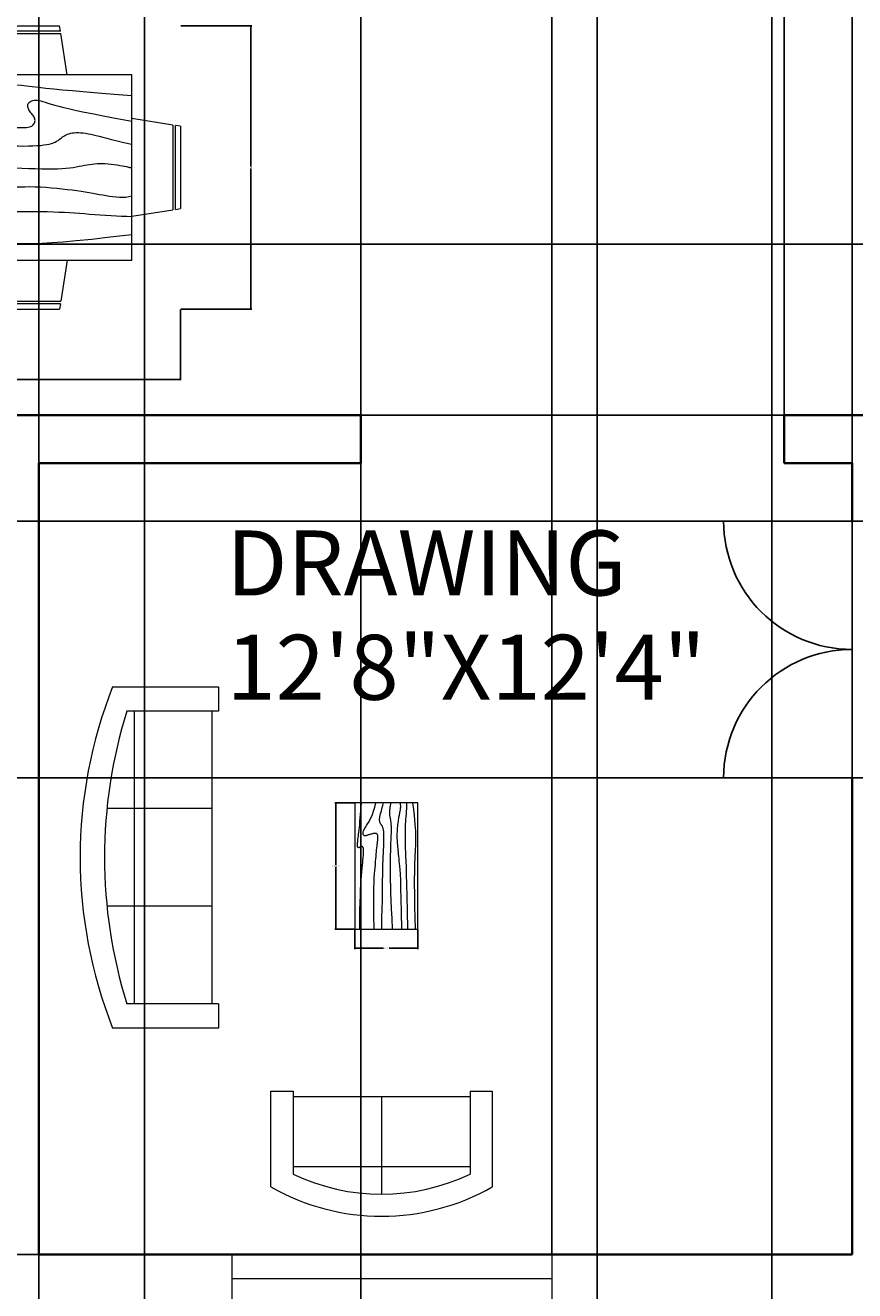
# Model space of a CAD drawing. Units: feet. Extents: x 2270 to 3094, y 1543 to 2352.
# Tile 4 of 6: x 2662 to 2817, y 1813 to 2050. Entities that reach past the tile are written whole.
import ezdxf

# ---------------------------------------------------------------- set-up
doc = ezdxf.new("R2010")
doc.units = ezdxf.units.FT
for name, color, linetype, lineweight in [('A-ANNO-DIMS', 2, 'Continuous', 18), ('A-AREA-IDEN', 7, 'Continuous', 18), ('A-DOOR', 3, 'Continuous', 25), ('A-FURN', 8, 'Continuous', 18), ('A-GLAZ', 4, 'Continuous', 18), ('A-WALL', 7, 'Continuous', 35)]:
    doc.layers.add(name, color=color, linetype=linetype, lineweight=lineweight)
doc.styles.get("Standard").update_dxf_attribs({"font": 'arial.ttf'})
doc.dimstyles.get("Standard").update_dxf_attribs({"dimtxt": 0.18, "dimasz": 0.18, "dimexe": 0.18, "dimexo": 0.0625, "dimgap": 0.09, "dimtad": 0, "dimtih": 1, "dimtoh": 1, "dimdec": 4, "dimzin": 0, "dimdsep": 46, "dimtxsty": 'Standard', "dimcen": 0.09, "dimadec": 0, "dimazin": 0, "dimtfac": 1, "dimtdec": 4, "dimtofl": 0, "dimtmove": 0, "dimatfit": 3, "dimfxl": 1, "dimtolj": 1, "dimtzin": 0, "dimarcsym": 0})

# ---------------------------------------------------------------- blocks, each defined once
blk = doc.blocks.new('Dining Set - 36 x 72 in.')
for p, q in [((-22, 27.5), (-22.1562, 26.50042)), ((-22, 27.5), (-6, 27.5)), ((-5.8437, 26.49966), (-6, 27.5)), ((6, 27.5), (5.8438, 26.50042)), ((6, 27.5), (22, 27.5)), ((22.1563, 26.49966), (22, 27.5)), ((-22.2343, 26.00059), (-23.4847, 17.99762)), ((-22.2304, 26), (-5.7608, 26)), ((-5.8416, 26.5), (-22.1534, 26.5)), ((-4.5152, 17.99762), (-5.7655, 25.99926)), ((5.7657, 26.00059), (4.5153, 17.99762)), ((5.7696, 26), (22.2392, 26)), ((22.1584, 26.5), (5.8466, 26.5)), ((23.4848, 17.99762), (22.2345, 25.99926)), ((36, 18), (-36, 18)), ((-36, 18), (-36, -18)), ((36, -18), (36, 18)), ((-45.5, 8), (-44.5004, 8.15617)), ((-45.5, 8), (-45.5, -8)), ((-44.5, -8.15843), (-44.5, 8.15338)), ((-44.0006, 8.23428), (-35.9976, 9.48474)), ((-44, 8.23041), (-44, -8.23915)), ((44.0006, 8.23428), (35.9976, 9.48474)), ((44, 8.23041), (44, -8.23915)), ((44.5, -8.15843), (44.5, 8.15338)), ((45.5, 8), (44.5005, 8.15617)), ((45.5, 8), (45.5, -8)), ((-44.4997, -8.15631), (-45.5, -8)), ((-35.9976, -9.48476), (-43.9993, -8.2345)), ((35.9976, -9.48476), (43.9993, -8.2345)), ((44.4997, -8.15631), (45.5, -8)), ((-36, -18), (36, -18)), ((-22.2343, -26.0006), (-23.4847, -17.99762)), ((-4.5152, -17.99762), (-5.7655, -25.99928)), ((5.7657, -26.0006), (4.5153, -17.99762)), ((23.4848, -17.99762), (22.2345, -25.99928)), ((-22.2304, -26), (-5.7608, -26)), ((-22, -27.5), (-22.1562, -26.50044)), ((-5.8416, -26.5), (-22.1534, -26.5)), ((-5.8437, -26.49967), (-6, -27.5)), ((5.7696, -26), (22.2392, -26)), ((6, -27.5), (5.8438, -26.50044)), ((22.1584, -26.5), (5.8466, -26.5)), ((22.1563, -26.49967), (22, -27.5)), ((-22, -27.5), (-6, -27.5)), ((6, -27.5), (22, -27.5))]:
    blk.add_line(p, q)
for points in [[(-36, 15), (-31.1772, 14.97754), (-26.8079, 14.91406), (-22.8538, 14.81543), (-19.276, 14.6875), (-16.0362, 14.53613), (-13.0957, 14.36718), (-10.4159, 14.18652), (-7.9583, 14), (-5.6904, 13.81315), (-3.6035, 13.63021), (-1.6954, 13.45508), (0.0365, 13.29166), (1.5945, 13.14388), (2.9811, 13.01562), (4.1988, 12.9108), (5.25, 12.83333), (6.1393, 12.78613), (6.8802, 12.76823), (7.4883, 12.77767), (7.9792, 12.8125), (8.3685, 12.87077), (8.6719, 12.95052), (8.9049, 13.0498), (9.0833, 13.16666), (9.2205, 13.29899), (9.3216, 13.44401), (9.3895, 13.59879), (9.4271, 13.76041), (9.4373, 13.92594), (9.4232, 14.09245), (9.3875, 14.257), (9.3333, 14.41666), (9.2638, 14.56917), (9.1836, 14.71484), (9.0975, 14.85465), (9.0104, 14.98958), (8.9272, 15.1206), (8.8529, 15.2487), (8.7922, 15.37483), (8.75, 15.5), (8.7305, 15.62467), (8.7344, 15.74739), (8.7617, 15.86621), (8.8125, 15.97916), (8.8867, 16.08431), (8.9844, 16.17968), (9.1055, 16.26334), (9.25, 16.33333), (9.4189, 16.38802), (9.6172, 16.42708), (9.8506, 16.45052), (10.125, 16.45833), (10.4463, 16.45052), (10.8203, 16.42708), (11.2529, 16.38802), (11.75, 16.33333), (12.3184, 16.26318), (12.9694, 16.17838), (13.7151, 16.07991), (14.5677, 15.96875), (15.5395, 15.84586), (16.6426, 15.71224), (17.8893, 15.56884), (19.2917, 15.41666), (20.859, 15.25667), (22.5879, 15.08984), (24.4721, 14.91715), (26.5052, 14.73958), (28.6809, 14.5581), (30.9929, 14.3737), (33.4347, 14.18733), (36, 14)], [(-36, 10), (-28.9766, 10.14274), (-23.1725, 10.20442), (-18.4241, 10.19775), (-14.5677, 10.13541), (-11.4399, 10.03011), (-8.877, 9.89453), (-6.7154, 9.74137), (-4.7917, 9.58333), (-2.9698, 9.43082), (-1.2246, 9.28515), (0.4415, 9.14534), (2.026, 9.01041), (3.5266, 8.87939), (4.9408, 8.7513), (6.266, 8.62516), (7.5, 8.5), (8.6411, 8.37549), (9.6914, 8.2539), (10.6538, 8.13818), (11.5312, 8.03125), (12.3267, 7.93603), (13.043, 7.85547), (13.6831, 7.79248), (14.25, 7.75), (14.7471, 7.7303), (15.1797, 7.73307), (15.5537, 7.75732), (15.875, 7.80208), (16.1494, 7.86637), (16.3828, 7.94922), (16.5811, 8.04964), (16.75, 8.16666), (16.8944, 8.29915), (17.0143, 8.44531), (17.1089, 8.60319), (17.1771, 8.77083), (17.218, 8.94629), (17.2305, 9.1276), (17.2137, 9.31282), (17.1667, 9.5), (17.0895, 9.6875), (16.987, 9.875), (16.8649, 10.0625), (16.7292, 10.25), (16.5856, 10.4375), (16.4401, 10.625), (16.2985, 10.8125), (16.1667, 11), (16.05, 11.18733), (15.9518, 11.3737), (15.8752, 11.5581), (15.8229, 11.73958), (15.798, 11.91715), (15.8034, 12.08984), (15.842, 12.25667), (15.9167, 12.41666), (16.0295, 12.56836), (16.1784, 12.70833), (16.3605, 12.83268), (16.5729, 12.9375), (16.8127, 13.01888), (17.0768, 13.07291), (17.3625, 13.0957), (17.6667, 13.08333), (17.9894, 13.03312), (18.3418, 12.94726), (18.7382, 12.82918), (19.1927, 12.68229), (19.7195, 12.51001), (20.3327, 12.31575), (21.0465, 12.10294), (21.875, 11.875), (22.8357, 11.63354), (23.959, 11.37304), (25.2786, 11.08618), (26.8282, 10.76562), (28.6414, 10.40405), (30.752, 9.99414), (33.1936, 9.52856), (36, 9)], [(-36, 5.5), (-30.7157, 5.3348), (-26.069, 5.20963), (-21.9946, 5.11767), (-18.4271, 5.05208), (-15.3009, 5.00602), (-12.5508, 4.97265), (-10.1112, 4.94515), (-7.9167, 4.91666), (-5.909, 4.88167), (-4.0586, 4.83984), (-2.3429, 4.79215), (-0.7396, 4.73958), (0.7739, 4.6831), (2.22, 4.6237), (3.6213, 4.56233), (5, 4.5), (6.373, 4.43782), (7.7344, 4.3776), (9.0723, 4.32129), (10.375, 4.27083), (11.6309, 4.22819), (12.8281, 4.19531), (13.9551, 4.17415), (15, 4.16666), (15.954, 4.17448), (16.819, 4.19791), (17.6001, 4.23698), (18.3021, 4.29166), (18.9299, 4.36198), (19.4883, 4.44791), (19.9823, 4.54948), (20.4167, 4.66666), (20.7969, 4.79899), (21.1302, 4.94401), (21.4245, 5.09879), (21.6875, 5.26041), (21.9271, 5.42594), (22.1511, 5.59245), (22.3672, 5.757), (22.5834, 5.91666), (22.8065, 6.06868), (23.0404, 6.21093), (23.2879, 6.34147), (23.5521, 6.45833), (23.8358, 6.55957), (24.142, 6.64323), (24.4735, 6.70735), (24.8334, 6.75), (25.2235, 6.76969), (25.642, 6.76692), (26.0858, 6.74267), (26.5521, 6.69791), (27.0379, 6.63362), (27.5404, 6.55078), (28.0565, 6.45036), (28.5834, 6.33333), (29.1242, 6.19987), (29.7071, 6.04687), (30.3661, 5.87044), (31.1354, 5.66666), (32.0493, 5.43164), (33.142, 5.16146), (34.4475, 4.85221), (36, 4.5)], [(-36, -1), (-30.7915, -0.6591), (-26.0195, -0.38216), (-21.6519, -0.16284), (-17.6563, 0.00521), (-14.0005, 0.12833), (-10.6523, 0.21289), (-7.5796, 0.26522), (-4.75, 0.29166), (-2.134, 0.29793), (0.2878, 0.28711), (2.5317, 0.26163), (4.6146, 0.22396), (6.5529, 0.17651), (8.3633, 0.12174), (10.0623, 0.06209), (11.6667, 0), (13.1899, -0.06201), (14.6341, -0.1211), (15.9982, -0.17432), (17.2813, -0.21875), (18.4823, -0.25147), (19.6003, -0.26953), (20.6343, -0.27002), (21.5834, -0.25), (22.4481, -0.20768), (23.2357, -0.14584), (23.9549, -0.06836), (24.6146, 0.02083), (25.2235, 0.11784), (25.7904, 0.21875), (26.3241, 0.31966), (26.8334, 0.41666), (27.3265, 0.50618), (27.8099, 0.58593), (28.2894, 0.65397), (28.7709, 0.70833), (29.2601, 0.74707), (29.763, 0.76823), (30.2855, 0.76985), (30.8334, 0.75), (31.4088, 0.70784), (31.9994, 0.64713), (32.589, 0.57275), (33.1615, 0.48958), (33.7008, 0.4025), (34.1908, 0.3164), (34.6153, 0.23616), (34.9584, 0.16666), (35.2099, 0.11165), (35.3848, 0.07031), (35.504, 0.04069), (35.5886, 0.02083), (35.6594, 0.00879), (35.7377, 0.0026), (35.8442, 0.00032), (36, 0)], [(-36, -6.5), (-27.1843, -6.31267), (-20.084, -6.1263), (-14.469, -5.9419), (-10.1094, -5.76042), (-6.7752, -5.58285), (-4.2363, -5.41016), (-2.2629, -5.24333), (-0.625, -5.08334), (0.8708, -4.93099), (2.2715, -4.78646), (3.5872, -4.64974), (4.8281, -4.52084), (6.0046, -4.39974), (7.127, -4.28646), (8.2053, -4.18099), (9.25, -4.08334), (10.2705, -3.99382), (11.2734, -3.91407), (12.2647, -3.84603), (13.25, -3.79167), (14.2354, -3.75293), (15.2266, -3.73177), (16.2295, -3.73015), (17.25, -3.75), (18.2912, -3.79248), (19.3451, -3.85547), (20.4009, -3.93604), (21.4479, -4.03125), (22.4754, -4.13819), (23.4727, -4.25391), (24.4289, -4.37549), (25.3334, -4.5), (26.1785, -4.62492), (26.9694, -4.74935), (27.7145, -4.87281), (28.4219, -4.99479), (29.1, -5.11483), (29.7572, -5.23242), (30.4016, -5.34709), (31.0417, -5.45834), (31.6837, -5.56437), (32.3262, -5.65821), (32.9658, -5.73153), (33.599, -5.77604), (34.2224, -5.78345), (34.8327, -5.74545), (35.4264, -5.65373), (36, -5.5)], [(-36, -10), (-26.4022, -9.81299), (-18.4675, -9.62891), (-11.9839, -9.45069), (-6.7396, -9.28125), (-2.5226, -9.12354), (0.8789, -8.98047), (3.6769, -8.85498), (6.0833, -8.75), (8.2767, -8.66765), (10.3021, -8.60677), (12.1712, -8.56543), (13.8958, -8.54167), (15.4876, -8.53353), (16.9583, -8.53907), (18.3197, -8.55632), (19.5834, -8.58334), (20.7616, -8.61841), (21.8685, -8.66081), (22.9188, -8.71004), (23.9271, -8.76563), (24.9081, -8.82707), (25.8763, -8.89388), (26.8465, -8.96558), (27.8334, -9.04167), (28.8474, -9.12118), (29.8828, -9.20117), (30.93, -9.27824), (31.9792, -9.34896), (33.0205, -9.40991), (34.0443, -9.45768), (35.0407, -9.48885), (36, -9.5)], [(-36, -14.5), (-30.0881, -14.33513), (-25.0332, -14.21224), (-20.7312, -14.12647), (-17.0781, -14.07292), (-13.97, -14.04671), (-11.3027, -14.04297), (-8.9724, -14.05681), (-6.875, -14.08334), (-4.9224, -14.11833), (-3.0905, -14.16016), (-1.3709, -14.20785), (0.2448, -14.26042), (1.7647, -14.3169), (3.1973, -14.3763), (4.5507, -14.43767), (5.8333, -14.5), (7.0554, -14.5621), (8.235, -14.62175), (9.3922, -14.67652), (10.5469, -14.72396), (11.7192, -14.76164), (12.929, -14.78711), (14.1965, -14.79794), (15.5417, -14.79167), (16.9933, -14.76424), (18.6152, -14.70508), (20.4804, -14.60197), (22.6615, -14.44271), (25.2312, -14.21509), (28.2624, -13.9069), (31.8277, -13.50594), (36, -13)]]:
    blk.add_lwpolyline(points)
blk = doc.blocks.new('Sofa - Roundback 7 ft.')
for p, q in [((-12.00002, -32.4421), (-12.00003, -6.5971)), ((11.99997, -32.4421), (11.99998, -6.5971)), ((-36.000027, -34), (-36.000027, -11.4696)), ((35.99998, -34), (35.99998, -11.4696)), ((-35.999844, -13.3819), (35.9998, -13.3819)), ((-36.000027, -32.4421), (35.99998, -32.4421))]:
    blk.add_line(p, q)
for points in [[(-36.000027, -34), (-42.000027, -34), (-42.000027, -8)], [(41.99998, -8), (41.99998, -34), (35.99998, -34)]]:
    blk.add_lwpolyline(points)
for centre, radius, start, end in [((0, -114.25), 114.25, 68.43141, 111.5686), ((-0.00001, -127.1968), 121.1968, 72.72033, 107.2797)]:
    blk.add_arc(centre, radius, start, end)
blk = doc.blocks.new('Sofa - Roundback Loveseat 5 ft.')
for p, q in [((0, -32.44198), (0, -5.99998)), ((-24, -33.99998), (-24, -11.46958)), ((-23.9998, -13.38178), (23.99986, -13.38178)), ((24.00004, -33.99998), (24.00004, -11.46958)), ((-24, -32.44198), (24.00004, -32.44198))]:
    blk.add_line(p, q)
for points in [[(-24, -33.99998), (-30, -33.99998), (-30, -7.99998)], [(30.00004, -7.99998), (30.00004, -33.99998), (24.00004, -33.99998)]]:
    blk.add_lwpolyline(points)
for centre, radius, start, end in [((0, -60.24998), 60.24998, 60.13715, 119.8628), ((0, -61.38438), 55.38444, 64.32083, 115.6792)]:
    blk.add_arc(centre, radius, start, end)
blk = doc.blocks.new('Table - Rectangular Woodgrain 60 x 30 in.')
for p, q in [((0, 0), (0, -30)), ((60, 0), (0, 0)), ((60, -30), (60, 0)), ((0, -30), (60, -30))]:
    blk.add_line(p, q)
for points in [[(0, -2.4), (4.8155, -2.418), (9.0302, -2.4688), (12.709, -2.5477), (15.9167, -2.65), (18.7181, -2.7711), (21.1781, -2.9063), (23.3616, -3.0508), (25.3333, -3.2), (27.1477, -3.3495), (28.8172, -3.4958), (30.3437, -3.636), (31.7291, -3.7667), (32.9756, -3.8849), (34.0849, -3.9875), (35.059, -4.0714), (35.9, -4.1334), (36.6114, -4.1711), (37.2041, -4.1854), (37.6906, -4.1779), (38.0833, -4.15), (38.3948, -4.1034), (38.6375, -4.0396), (38.8239, -3.9602), (38.9666, -3.8667), (39.0764, -3.7608), (39.1573, -3.6448), (39.2116, -3.521), (39.2416, -3.3917), (39.2498, -3.2593), (39.2385, -3.1261), (39.21, -2.9944), (39.1666, -2.8667), (39.111, -2.7447), (39.0468, -2.6281), (38.978, -2.5163), (38.9083, -2.4083), (38.8418, -2.3035), (38.7823, -2.201), (38.7337, -2.1001), (38.7, -2), (38.6844, -1.9003), (38.6875, -1.8021), (38.7094, -1.707), (38.75, -1.6167), (38.8094, -1.5326), (38.8875, -1.4563), (38.9844, -1.3893), (39.1, -1.3333), (39.2351, -1.2896), (39.3937, -1.2583), (39.5804, -1.2396), (39.8, -1.2333), (40.057, -1.2396), (40.3562, -1.2583), (40.7023, -1.2896), (41.1, -1.3333), (41.5547, -1.3895), (42.0755, -1.4573), (42.6721, -1.5361), (43.3542, -1.625), (44.1316, -1.7233), (45.014, -1.8302), (46.0114, -1.9449), (47.1333, -2.0667), (48.3862, -2.1947), (49.7625, -2.3281), (51.2513, -2.4663), (52.8416, -2.6083), (54.5226, -2.7535), (56.2833, -2.9011), (58.1127, -3.0501), (60, -3.2)], [(0, -9.2), (6.5759, -9.0858), (11.9385, -9.0365), (16.2527, -9.0418), (19.6833, -9.0917), (22.3952, -9.1759), (24.5531, -9.2844), (26.322, -9.4069), (27.8666, -9.5333), (29.3241, -9.6553), (30.7203, -9.7719), (32.0532, -9.8837), (33.3208, -9.9917), (34.5213, -10.0965), (35.6526, -10.199), (36.7128, -10.2999), (37.7, -10.4), (38.6129, -10.4996), (39.4531, -10.5969), (40.223, -10.6895), (40.925, -10.775), (41.5613, -10.8512), (42.1344, -10.9156), (42.6465, -10.966), (43.1, -11), (43.4976, -11.0158), (43.8437, -11.0136), (44.143, -10.9942), (44.4, -10.9583), (44.6195, -10.9069), (44.8062, -10.8406), (44.9648, -10.7603), (45.1, -10.6667), (45.2155, -10.5598), (45.3114, -10.4365), (45.3871, -10.2929), (45.4416, -10.125), (45.4743, -9.929), (45.4844, -9.7011), (45.4709, -9.4371), (45.4333, -9.1333), (45.3716, -8.7883), (45.2896, -8.4104), (45.1919, -8.0107), (45.0833, -7.6), (44.9685, -7.1893), (44.8521, -6.7896), (44.7388, -6.4117), (44.6333, -6.0667), (44.54, -5.7628), (44.4614, -5.4979), (44.4001, -5.2675), (44.3583, -5.0667), (44.3384, -4.8909), (44.3427, -4.7354), (44.3736, -4.5956), (44.4333, -4.4667), (44.5236, -4.3453), (44.6427, -4.2333), (44.7884, -4.1339), (44.9583, -4.05), (45.1501, -3.9849), (45.3614, -3.9417), (45.59, -3.9234), (45.8333, -3.9333), (46.0915, -3.9749), (46.3734, -4.0531), (46.6906, -4.1736), (47.0542, -4.3417), (47.4756, -4.5629), (47.9661, -4.8427), (48.5372, -5.1866), (49.2, -5.6), (49.9676, -6.0844), (50.8594, -6.625), (51.8965, -7.2031), (53.1, -7.8), (54.491, -8.3969), (56.0906, -8.975), (57.9199, -9.5156), (60, -10)], [(0, -12.8), (5.1847, -12.9322), (9.6213, -13.0323), (13.3963, -13.1059), (16.5958, -13.1583), (19.3063, -13.1952), (21.614, -13.2219), (23.6054, -13.2439), (25.3666, -13.2667), (26.9728, -13.2947), (28.4531, -13.3281), (29.8256, -13.3663), (31.1083, -13.4083), (32.3191, -13.4535), (33.476, -13.501), (34.597, -13.5501), (35.7, -13.6), (36.7984, -13.6497), (37.8875, -13.6979), (38.9578, -13.743), (40, -13.7833), (41.0047, -13.8174), (41.9625, -13.8438), (42.864, -13.8607), (43.7, -13.8667), (44.4631, -13.8604), (45.1552, -13.8417), (45.7801, -13.8104), (46.3416, -13.7667), (46.8439, -13.7104), (47.2906, -13.6417), (47.6858, -13.5604), (48.0333, -13.4667), (48.3375, -13.3608), (48.6042, -13.2448), (48.8396, -13.121), (49.05, -12.9917), (49.2417, -12.8593), (49.4208, -12.7261), (49.5937, -12.5944), (49.7667, -12.4667), (49.9452, -12.3451), (50.1323, -12.2313), (50.3303, -12.1268), (50.5416, -12.0333), (50.7686, -11.9524), (51.0135, -11.8854), (51.2788, -11.8341), (51.5666, -11.8), (51.8785, -11.7843), (52.2116, -11.7865), (52.562, -11.8059), (52.926, -11.8417), (53.2998, -11.8931), (53.6795, -11.9594), (54.0614, -12.0397), (54.4416, -12.1333), (54.8223, -12.2401), (55.2293, -12.3625), (55.6942, -12.5037), (56.2489, -12.6667), (56.9251, -12.8547), (57.7545, -13.0708), (58.7689, -13.3182), (60, -13.6)], [(0, -18), (5.124, -17.7273), (9.6609, -17.5057), (13.6705, -17.3303), (17.2125, -17.1958), (20.3467, -17.0973), (23.1328, -17.0297), (25.6307, -16.9878), (27.9, -16.9667), (29.9928, -16.9617), (31.9302, -16.9703), (33.7254, -16.9907), (35.3917, -17.0208), (36.9423, -17.0588), (38.3906, -17.1026), (39.7499, -17.1503), (41.0333, -17.2), (42.2519, -17.2496), (43.4073, -17.2969), (44.4986, -17.3395), (45.525, -17.375), (46.4858, -17.4012), (47.3802, -17.4156), (48.2074, -17.416), (48.9667, -17.4), (49.6583, -17.3662), (50.2872, -17.3167), (50.8595, -17.2547), (51.3812, -17.1833), (51.8584, -17.1057), (52.2971, -17.025), (52.7034, -16.9443), (53.0833, -16.8667), (53.443, -16.7951), (53.789, -16.7313), (54.128, -16.6768), (54.4666, -16.6334), (54.8115, -16.6024), (55.1693, -16.5854), (55.5465, -16.5841), (55.95, -16.6), (56.3828, -16.6337), (56.8346, -16.6823), (57.2915, -16.7418), (57.7396, -16.8084), (58.165, -16.878), (58.5539, -16.9469), (58.8924, -17.0111), (59.1666, -17.0667), (59.3679, -17.1107), (59.5078, -17.1438), (59.6032, -17.1675), (59.6708, -17.1833), (59.7275, -17.193), (59.7901, -17.1979), (59.8753, -17.1998), (60, -17.2)], [(0, -22.4), (8.0098, -22.2501), (14.4094, -22.1011), (19.4168, -21.9535), (23.25, -21.8083), (26.1269, -21.6663), (28.2656, -21.5281), (29.884, -21.3947), (31.2, -21.2667), (32.3967, -21.1448), (33.5172, -21.0292), (34.5697, -20.9198), (35.5625, -20.8167), (36.5037, -20.7198), (37.4015, -20.6292), (38.2642, -20.5448), (39.1, -20.4667), (39.9164, -20.3951), (40.7187, -20.3313), (41.5117, -20.2768), (42.3, -20.2333), (43.0883, -20.2024), (43.8812, -20.1854), (44.6836, -20.1841), (45.5, -20.2), (46.3328, -20.234), (47.1747, -20.2844), (48.0163, -20.3488), (48.8479, -20.425), (49.66, -20.5106), (50.4429, -20.6031), (51.1872, -20.7004), (51.8833, -20.8), (52.5246, -20.8999), (53.1166, -20.9995), (53.6681, -21.0983), (54.1875, -21.1958), (54.6834, -21.2919), (55.1646, -21.3859), (55.6394, -21.4777), (56.1167, -21.5667), (56.6028, -21.6515), (57.0961, -21.7266), (57.5929, -21.7852), (58.0896, -21.8208), (58.5823, -21.8268), (59.0674, -21.7964), (59.5412, -21.723), (60, -21.6)], [(0, -25.2), (8.6355, -25.0504), (15.7026, -24.9031), (21.4049, -24.7606), (25.9458, -24.625), (29.529, -24.4988), (32.3578, -24.3844), (34.6359, -24.284), (36.5667, -24.2), (38.3213, -24.1341), (39.9417, -24.0854), (41.437, -24.0523), (42.8167, -24.0333), (44.0901, -24.0268), (45.2667, -24.0313), (46.3557, -24.0451), (47.3667, -24.0667), (48.309, -24.0947), (49.1928, -24.1287), (50.0284, -24.168), (50.826, -24.2125), (51.5959, -24.2617), (52.3483, -24.3151), (53.0935, -24.3725), (53.8417, -24.4334), (54.6009, -24.497), (55.3699, -24.561), (56.1454, -24.6226), (56.9239, -24.6792), (57.7021, -24.7279), (58.4764, -24.7662), (59.2435, -24.7911), (60, -24.8)], [(0, -28.8), (5.6867, -28.6681), (10.45, -28.5698), (14.407, -28.5012), (17.675, -28.4584), (20.3711, -28.4374), (22.6125, -28.4344), (24.5164, -28.4455), (26.2, -28.4667), (27.762, -28.4947), (29.2276, -28.5281), (30.6033, -28.5663), (31.8958, -28.6084), (33.1118, -28.6535), (34.2578, -28.7011), (35.3405, -28.7501), (36.3666, -28.8), (37.3443, -28.8497), (38.288, -28.8974), (39.2137, -28.9412), (40.1375, -28.9792), (41.0753, -29.0093), (42.0432, -29.0297), (43.0572, -29.0384), (44.1333, -29.0333), (45.2936, -29.0114), (46.5843, -28.9641), (48.0579, -28.8816), (49.7666, -28.7542), (51.7629, -28.5721), (54.0989, -28.3255), (56.8272, -28.0048), (60, -27.6)]]:
    blk.add_lwpolyline(points)
blk = doc.blocks.new('DOOR-SWING-24')
blk.add_line((33, 0), (0, 0))
blk.add_arc((9, 0), 24, 0, 90)
blk = doc.blocks.new('*D22')
at = {"layer": 'A-ANNO-DIMS', "color": 0, "lineweight": -2, "transparency": 16777216}
for p, q in [((2723.65, 1904.57), (2719.99, 1904.57)), ((2720.17, 1904.39), (2720.17, 1892.94)), ((2720.17, 1881.13), (2720.17, 1892.58)), ((2723.65, 1880.95), (2719.99, 1880.95))]:
    blk.add_line(p, q, dxfattribs=at)
at = {"layer": 'A-ANNO-DIMS', "color": 0, "transparency": 16777216}
for points in [[(2720.14, 1904.39), (2720.2, 1904.39), (2720.17, 1904.57)], [(2720.14, 1881.13), (2720.2, 1881.13), (2720.17, 1880.95)]]:
    blk.add_solid(points, dxfattribs=at)
at = {"layer": 'Defpoints', "color": 0, "transparency": 16777216}
for p in [(2720.17, 1904.57), (2723.71, 1904.57), (2723.71, 1880.95)]:
    blk.add_point(p, dxfattribs=at)
at = {"layer": 'A-ANNO-DIMS', "color": 0, "transparency": 16777216, "insert": (2720.17, 1892.76), "char_height": 0.18, "attachment_point": 5}
blk.add_mtext('\\A1;TABLE 24 TYP.', dxfattribs=at)
blk = doc.blocks.new('*D23')
at = {"layer": 'A-ANNO-DIMS', "color": 0, "lineweight": -2, "transparency": 16777216}
for p, q in [((2723.71, 1880.89), (2723.71, 1877.23)), ((2735.52, 1880.89), (2735.52, 1877.23)), ((2723.89, 1877.41), (2729.09, 1877.41)), ((2735.34, 1877.41), (2730.13, 1877.41))]:
    blk.add_line(p, q, dxfattribs=at)
at = {"layer": 'A-ANNO-DIMS', "color": 0, "transparency": 16777216}
for points in [[(2723.89, 1877.44), (2723.89, 1877.38), (2723.71, 1877.41)], [(2735.34, 1877.44), (2735.34, 1877.38), (2735.52, 1877.41)]]:
    blk.add_solid(points, dxfattribs=at)
at = {"layer": 'Defpoints', "color": 0, "transparency": 16777216}
for p in [(2723.71, 1880.95), (2735.52, 1880.95), (2723.71, 1877.41)]:
    blk.add_point(p, dxfattribs=at)
at = {"layer": 'A-ANNO-DIMS', "color": 0, "transparency": 16777216, "insert": (2729.61, 1877.41), "char_height": 0.18, "attachment_point": 5}
blk.add_mtext('\\A1;12 TYP.', dxfattribs=at)
blk = doc.blocks.new('*D24')
at = {"layer": 'A-ANNO-DIMS', "color": 0, "lineweight": -2, "transparency": 16777216}
for p, q in [((2603.54, 1996.85), (2603.54, 1983.59)), ((2691.16, 1996.85), (2691.16, 1983.59)), ((2603.72, 1983.77), (2646.38, 1983.77)), ((2690.98, 1983.77), (2648.32, 1983.77))]:
    blk.add_line(p, q, dxfattribs=at)
at = {"layer": 'A-ANNO-DIMS', "color": 0, "transparency": 16777216}
for points in [[(2603.72, 1983.8), (2603.72, 1983.74), (2603.54, 1983.77)], [(2690.98, 1983.8), (2690.98, 1983.74), (2691.16, 1983.77)]]:
    blk.add_solid(points, dxfattribs=at)
at = {"layer": 'Defpoints', "color": 0, "transparency": 16777216}
for p in [(2603.54, 1996.92), (2691.16, 1996.92), (2691.16, 1983.77)]:
    blk.add_point(p, dxfattribs=at)
at = {"layer": 'A-ANNO-DIMS', "color": 0, "transparency": 16777216, "insert": (2647.35, 1983.77), "char_height": 0.18, "attachment_point": 5}
blk.add_mtext('\\A1;DINING SET 88', dxfattribs=at)
blk = doc.blocks.new('*D25')
at = {"layer": 'A-ANNO-DIMS', "color": 0, "lineweight": -2, "transparency": 16777216}
for p, q in [((2691.22, 2049.87), (2704.48, 2049.87)), ((2704.3, 2049.69), (2704.3, 2023.58)), ((2704.3, 1997.1), (2704.3, 2023.21)), ((2691.22, 1996.92), (2704.48, 1996.92))]:
    blk.add_line(p, q, dxfattribs=at)
at = {"layer": 'A-ANNO-DIMS', "color": 0, "transparency": 16777216}
for points in [[(2704.27, 2049.69), (2704.33, 2049.69), (2704.3, 2049.87)], [(2704.27, 1997.1), (2704.33, 1997.1), (2704.3, 1996.92)]]:
    blk.add_solid(points, dxfattribs=at)
at = {"layer": 'Defpoints', "color": 0, "transparency": 16777216}
for p in [(2691.16, 2049.87), (2704.3, 2049.87), (2691.16, 1996.92)]:
    blk.add_point(p, dxfattribs=at)
at = {"layer": 'A-ANNO-DIMS', "color": 0, "transparency": 16777216, "insert": (2704.3, 2023.4), "char_height": 0.18, "attachment_point": 5}
blk.add_mtext('\\A1;53', dxfattribs=at)
blk = doc.blocks.new('*D36')
at = {"layer": 'A-ANNO-DIMS', "color": 0, "lineweight": -2, "transparency": 16777216}
for p, q in [((2652.67, 2243.02), (2652.67, 1574.6)), ((2684.42, 2243.02), (2684.42, 1574.6)), ((2652.85, 1574.78), (2668.15, 1574.78)), ((2684.24, 1574.78), (2668.94, 1574.78))]:
    blk.add_line(p, q, dxfattribs=at)
at = {"layer": 'A-ANNO-DIMS', "color": 0, "transparency": 16777216}
for points in [[(2652.85, 1574.81), (2652.85, 1574.75), (2652.67, 1574.78)], [(2684.24, 1574.81), (2684.24, 1574.75), (2684.42, 1574.78)]]:
    blk.add_solid(points, dxfattribs=at)
at = {"layer": 'Defpoints', "color": 0, "transparency": 16777216}
for p in [(2652.67, 2243.08), (2684.42, 2243.08), (2684.42, 1574.78)]:
    blk.add_point(p, dxfattribs=at)
at = {"layer": 'A-ANNO-DIMS', "color": 0, "transparency": 16777216, "insert": (2668.55, 1574.78), "char_height": 0.18, "attachment_point": 5}
blk.add_mtext('\\A1;31.76', dxfattribs=at)
blk = doc.blocks.new('*D37')
at = {"layer": 'A-ANNO-DIMS', "color": 0, "lineweight": -2, "transparency": 16777216}
for p, q in [((2684.42, 2243.02), (2684.42, 1574.6)), ((2769.01, 2243.02), (2769.01, 1574.6)), ((2684.6, 1574.78), (2726.32, 1574.78)), ((2768.83, 1574.78), (2727.11, 1574.78))]:
    blk.add_line(p, q, dxfattribs=at)
at = {"layer": 'A-ANNO-DIMS', "color": 0, "transparency": 16777216}
for points in [[(2684.6, 1574.81), (2684.6, 1574.75), (2684.42, 1574.78)], [(2768.83, 1574.81), (2768.83, 1574.75), (2769.01, 1574.78)]]:
    blk.add_solid(points, dxfattribs=at)
at = {"layer": 'Defpoints', "color": 0, "transparency": 16777216}
for p in [(2684.42, 2243.08), (2769.01, 2243.08), (2769.01, 1574.78)]:
    blk.add_point(p, dxfattribs=at)
at = {"layer": 'A-ANNO-DIMS', "color": 0, "transparency": 16777216, "insert": (2726.71, 1574.78), "char_height": 0.18, "attachment_point": 5}
blk.add_mtext('\\A1;84.58', dxfattribs=at)
blk = doc.blocks.new('*D44')
at = {"layer": 'A-ANNO-DIMS', "color": 0, "lineweight": -2, "transparency": 16777216}
for p, q in [((2816.6, 1957.26), (2270.19, 1957.26)), ((2270.37, 1957.08), (2270.37, 1933.44)), ((2270.37, 1909.44), (2270.37, 1933.08)), ((2816.6, 1909.26), (2270.19, 1909.26))]:
    blk.add_line(p, q, dxfattribs=at)
at = {"layer": 'A-ANNO-DIMS', "color": 0, "transparency": 16777216}
for points in [[(2270.34, 1957.08), (2270.4, 1957.08), (2270.37, 1957.26)], [(2270.34, 1909.44), (2270.4, 1909.44), (2270.37, 1909.26)]]:
    blk.add_solid(points, dxfattribs=at)
at = {"layer": 'Defpoints', "color": 0, "transparency": 16777216}
for p in [(2270.37, 1957.26), (2816.67, 1957.26), (2816.67, 1909.26)]:
    blk.add_point(p, dxfattribs=at)
at = {"layer": 'A-ANNO-DIMS', "color": 0, "transparency": 16777216, "insert": (2270.37, 1933.26), "char_height": 0.18, "attachment_point": 5}
blk.add_mtext('\\A1;48', dxfattribs=at)
blk = doc.blocks.new('*D45')
at = {"layer": 'A-ANNO-DIMS', "color": 0, "lineweight": -2, "transparency": 16777216}
for p, q in [((2816.6, 1909.26), (2270.19, 1909.26)), ((2270.37, 1909.08), (2270.37, 1864.85)), ((2270.37, 1820.26), (2270.37, 1864.49)), ((2816.6, 1820.08), (2270.19, 1820.08))]:
    blk.add_line(p, q, dxfattribs=at)
at = {"layer": 'A-ANNO-DIMS', "color": 0, "transparency": 16777216}
for points in [[(2270.34, 1909.08), (2270.4, 1909.08), (2270.37, 1909.26)], [(2270.34, 1820.26), (2270.4, 1820.26), (2270.37, 1820.08)]]:
    blk.add_solid(points, dxfattribs=at)
at = {"layer": 'Defpoints', "color": 0, "transparency": 16777216}
for p in [(2270.37, 1909.26), (2816.67, 1909.26), (2816.67, 1820.08)]:
    blk.add_point(p, dxfattribs=at)
at = {"layer": 'A-ANNO-DIMS', "color": 0, "transparency": 16777216, "insert": (2270.37, 1864.67), "char_height": 0.18, "attachment_point": 5}
blk.add_mtext('\\A1;89.18', dxfattribs=at)
blk = doc.blocks.new('*D47')
at = {"layer": 'A-ANNO-DIMS', "color": 0, "lineweight": -2, "transparency": 16777216}
for p, q in [((2760.54, 1820.15), (2760.54, 2351.56)), ((2760.72, 2351.38), (2788.21, 2351.38)), ((2816.49, 2351.38), (2788.99, 2351.38)), ((2816.67, 1820.15), (2816.67, 2351.56))]:
    blk.add_line(p, q, dxfattribs=at)
at = {"layer": 'A-ANNO-DIMS', "color": 0, "transparency": 16777216}
for points in [[(2760.72, 2351.41), (2760.72, 2351.35), (2760.54, 2351.38)], [(2816.49, 2351.41), (2816.49, 2351.35), (2816.67, 2351.38)]]:
    blk.add_solid(points, dxfattribs=at)
at = {"layer": 'Defpoints', "color": 0, "transparency": 16777216}
for p in [(2816.67, 2351.38), (2760.54, 1820.08), (2816.67, 1820.08)]:
    blk.add_point(p, dxfattribs=at)
at = {"layer": 'A-ANNO-DIMS', "color": 0, "transparency": 16777216, "insert": (2788.6, 2351.38), "char_height": 0.18, "attachment_point": 5}
blk.add_mtext('\\A1;56.13', dxfattribs=at)
blk = doc.blocks.new('*D48')
at = {"layer": 'A-ANNO-DIMS', "color": 0, "lineweight": -2, "transparency": 16777216}
for p, q in [((2664.67, 1698.15), (2664.67, 2351.56)), ((2664.85, 2351.38), (2732.89, 2351.38)), ((2801.49, 2351.38), (2733.45, 2351.38)), ((2801.67, 1698.15), (2801.67, 2351.56))]:
    blk.add_line(p, q, dxfattribs=at)
at = {"layer": 'A-ANNO-DIMS', "color": 0, "transparency": 16777216}
for points in [[(2664.85, 2351.41), (2664.85, 2351.35), (2664.67, 2351.38)], [(2801.49, 2351.41), (2801.49, 2351.35), (2801.67, 2351.38)]]:
    blk.add_solid(points, dxfattribs=at)
at = {"layer": 'Defpoints', "color": 0, "transparency": 16777216}
for p in [(2801.67, 2351.38), (2664.67, 1698.08), (2801.67, 1698.08)]:
    blk.add_point(p, dxfattribs=at)
at = {"layer": 'A-ANNO-DIMS', "color": 0, "transparency": 16777216, "insert": (2733.17, 2351.38), "char_height": 0.18, "attachment_point": 5}
blk.add_mtext('\\A1;137', dxfattribs=at)
blk = doc.blocks.new('*D56')
at = {"layer": 'A-ANNO-DIMS', "color": 0, "lineweight": -2, "transparency": 16777216}
for p, q in [((2378.73, 2009.08), (3094.15, 2009.08)), ((3093.97, 2008.9), (3093.97, 1993.27)), ((3093.97, 1977.26), (3093.97, 1992.9)), ((2378.73, 1977.08), (3094.15, 1977.08))]:
    blk.add_line(p, q, dxfattribs=at)
at = {"layer": 'A-ANNO-DIMS', "color": 0, "transparency": 16777216}
for points in [[(3093.94, 2008.9), (3094, 2008.9), (3093.97, 2009.08)], [(3093.94, 1977.26), (3094, 1977.26), (3093.97, 1977.08)]]:
    blk.add_solid(points, dxfattribs=at)
at = {"layer": 'Defpoints', "color": 0, "transparency": 16777216}
for p in [(2378.67, 2009.08), (3093.97, 2009.08), (2378.67, 1977.08)]:
    blk.add_point(p, dxfattribs=at)
at = {"layer": 'A-ANNO-DIMS', "color": 0, "transparency": 16777216, "insert": (3093.97, 1993.08), "char_height": 0.18, "attachment_point": 5}
blk.add_mtext('\\A1;32', dxfattribs=at)
blk = doc.blocks.new('*D66')
at = {"layer": 'A-ANNO-DIMS', "color": 0, "lineweight": -2, "transparency": 16777216}
for p, q in [((2724.84, 1977.15), (2724.84, 2351.56)), ((2725.02, 2351.38), (2764.01, 2351.38)), ((2803.78, 2351.38), (2764.79, 2351.38)), ((2803.96, 1977.15), (2803.96, 2351.56))]:
    blk.add_line(p, q, dxfattribs=at)
at = {"layer": 'A-ANNO-DIMS', "color": 0, "transparency": 16777216}
for points in [[(2725.02, 2351.41), (2725.02, 2351.35), (2724.84, 2351.38)], [(2803.78, 2351.41), (2803.78, 2351.35), (2803.96, 2351.38)]]:
    blk.add_solid(points, dxfattribs=at)
at = {"layer": 'Defpoints', "color": 0, "transparency": 16777216}
for p in [(2803.96, 2351.38), (2724.84, 1977.08), (2803.96, 1977.08)]:
    blk.add_point(p, dxfattribs=at)
at = {"layer": 'A-ANNO-DIMS', "color": 0, "transparency": 16777216, "insert": (2764.4, 2351.38), "char_height": 0.18, "attachment_point": 5}
blk.add_mtext('\\A1;79.12', dxfattribs=at)
blk = doc.blocks.new('*D67')
at = {"layer": 'A-ANNO-DIMS', "color": 0, "lineweight": -2, "transparency": 16777216}
for p, q in [((2664.67, 1968.02), (2664.67, 1574.6)), ((2724.84, 1968.02), (2724.84, 1574.6)), ((2664.85, 1574.78), (2694.36, 1574.78)), ((2724.66, 1574.78), (2695.15, 1574.78))]:
    blk.add_line(p, q, dxfattribs=at)
at = {"layer": 'A-ANNO-DIMS', "color": 0, "transparency": 16777216}
for points in [[(2664.85, 1574.81), (2664.85, 1574.75), (2664.67, 1574.78)], [(2724.66, 1574.81), (2724.66, 1574.75), (2724.84, 1574.78)]]:
    blk.add_solid(points, dxfattribs=at)
at = {"layer": 'Defpoints', "color": 0, "transparency": 16777216}
for p in [(2664.67, 1968.08), (2724.84, 1968.08), (2664.67, 1574.78)]:
    blk.add_point(p, dxfattribs=at)
at = {"layer": 'A-ANNO-DIMS', "color": 0, "transparency": 16777216, "insert": (2694.75, 1574.78), "char_height": 0.18, "attachment_point": 5}
blk.add_mtext('\\A1;60.17', dxfattribs=at)

msp = doc.modelspace()

# ---------------------------------------------------------------- linework, layer by layer
at = {"layer": 'A-DOOR'}
for q in [(2792.6659, 1957.2599), (2825.6659, 1957.2599)]:
    msp.add_line((2816.6659, 1957.2599), q, dxfattribs=at)
msp.add_arc((2816.6659, 1957.2599), 24, 180, 270, dxfattribs=at)
at = {"layer": 'A-GLAZ'}
for p, q in [((2700.7017, 1820.0845), (2700.7017, 1811.0845)), ((2760.5365, 1820.0845), (2760.5365, 1811.0845)), ((2700.7017, 1815.5845), (2760.5365, 1815.5845))]:
    msp.add_line(p, q, dxfattribs=at)
at = {"layer": 'A-WALL'}
for p, q in [((2598.6659, 1977.0845), (2724.8399, 1977.0845)), ((2724.8399, 1977.0845), (2724.8399, 1968.0845)), ((2803.9581, 1977.0845), (2803.9581, 1968.0845)), ((2803.9581, 1977.0845), (2885.6659, 1977.0845)), ((2664.6659, 1968.0845), (2664.6659, 1820.0845)), ((2664.6659, 1968.0845), (2724.8399, 1968.0845)), ((2803.9581, 1968.0845), (2816.6659, 1968.0845)), ((2816.6659, 1968.0845), (2816.6659, 1957.2599)), ((2816.6659, 1909.2599), (2816.6659, 1820.0845)), ((2816.6659, 1820.0845), (2664.6659, 1820.0845))]:
    msp.add_line(p, q, dxfattribs=at)

# ---------------------------------------------------------------- block references
at = {"layer": 'A-DOOR', "extrusion": (0, 0, -1), "zscale": -1}
msp.add_blockref('DOOR-SWING-24', (-2825.6658, 1909.2604), dxfattribs=at)
at = {"layer": 'A-FURN', "xscale": 0.96282654590751, "yscale": 0.96282654590751, "zscale": 0.96282654590751}
msp.add_blockref('Dining Set - 36 x 72 in.', (2647.3519, 2023.3951), dxfattribs=at)
at = {"layer": 'A-FURN'}
for name, p, xscale, yscale, zscale, rotation in [('Sofa - Roundback 7 ft.', (2672.3653, 1894.3709), 0.7600860967180219, 0.7600860967180219, 0.7600860967180219, 89.99997783100054), ('Table - Rectangular Woodgrain 60 x 30 in.', (2723.7093, 1880.9531), 0.3935928378760143, 0.3935928378760143, 0.3935928378760143, 90), ('Sofa - Roundback Loveseat 5 ft.', (2728.7196, 1827.251), 0.6890107561229493, 0.6890107561229493, 0.6890107561229493, 180)]:
    msp.add_blockref(name, p, dxfattribs=dict(at, xscale=xscale, yscale=yscale, zscale=zscale, rotation=rotation))

# ---------------------------------------------------------------- texts
at = {"layer": 'A-AREA-IDEN'}
for s, height, p in [('DRAWING', 12.14556, (2699.7187, 1943.3565)), ('12\'8"X12\'4"', 12.145557, (2699.7187, 1923.8458))]:
    msp.add_text(s, height=height, dxfattribs=at).set_placement(p)

# ---------------------------------------------------------------- dimensions: what is measured, and where the dimension line sits
at = {"layer": 'A-ANNO-DIMS'}
for base, p1, p2, override, picture, middle in [((2801.6659, 2351.3845), (2664.6659, 1698.0845), (2801.6659, 1698.0845), {"dimdec": 0, "dimlfac": 1, "dimrnd": 0, "dimzin": 0, "dimdsep": 46, "dimlunit": 2}, '*D48', (2733.1659, 2351.3845)), ((2803.9581, 2351.3845), (2724.8399, 1977.0845), (2803.9581, 1977.0845), {"dimdec": 2, "dimlfac": 1, "dimrnd": 0, "dimzin": 0, "dimdsep": 46, "dimlunit": 2}, '*D66', (2764.399, 2351.3845)), ((2816.6659, 2351.3845), (2760.5365, 1820.0845), (2816.6659, 1820.0845), {"dimdec": 2, "dimlfac": 1, "dimrnd": 0, "dimzin": 0, "dimdsep": 46, "dimlunit": 2}, '*D47', (2788.6012, 2351.3845)), ((2684.4243, 1574.7845), (2652.6659, 2243.0845), (2684.4243, 2243.0845), {"dimdec": 2, "dimlfac": 1, "dimrnd": 0, "dimzin": 0, "dimdsep": 46, "dimlunit": 2}, '*D36', (2668.5451, 1574.7845)), ((2769.0053, 1574.7845), (2684.4243, 2243.0845), (2769.0053, 2243.0845), {"dimdec": 2, "dimlfac": 1, "dimrnd": 0, "dimzin": 0, "dimdsep": 46, "dimlunit": 2}, '*D37', (2726.7148, 1574.7845)), ((2664.6659, 1574.7845), (2724.8399, 1968.0845), (2664.6659, 1968.0845), {"dimdec": 2, "dimlfac": 1, "dimrnd": 0, "dimzin": 0, "dimdsep": 46, "dimlunit": 2}, '*D67', (2694.7529, 1574.7845))]:
    dim = msp.add_linear_dim(base=base, p1=p1, p2=p2, dimstyle='Standard', override=override, dxfattribs=at)
    dim.commit()
    dim.dimension.update_dxf_attribs({"geometry": picture, "text_midpoint": middle})
for base, p1, p2, override, picture, middle in [((2704.3031, 2049.8729), (2691.1605, 1996.9174), (2691.1605, 2049.8729), {"dimdec": 0, "dimlfac": 1, "dimrnd": 0, "dimzin": 0, "dimdsep": 46, "dimlunit": 2}, '*D25', (2704.3031, 2023.3951)), ((3093.9659, 2009.0845), (2378.6659, 1977.0845), (2378.6659, 2009.0845), {"dimdec": 0, "dimlfac": 1, "dimrnd": 0, "dimzin": 0, "dimdsep": 46, "dimlunit": 2}, '*D56', (3093.9659, 1993.0845)), ((2270.3659, 1957.2599), (2816.6659, 1909.2599), (2816.6659, 1957.2599), {"dimdec": 0, "dimlfac": 1, "dimrnd": 0, "dimzin": 0, "dimdsep": 46, "dimlunit": 2}, '*D44', (2270.3659, 1933.2599)), ((2270.3659, 1909.2599), (2816.6659, 1820.0845), (2816.6659, 1909.2599), {"dimdec": 2, "dimlfac": 1, "dimrnd": 0, "dimzin": 0, "dimdsep": 46, "dimlunit": 2}, '*D45', (2270.3659, 1864.6722))]:
    dim = msp.add_linear_dim(base=base, p1=p1, p2=p2, angle=90, dimstyle='Standard', override=override, dxfattribs=at)
    dim.commit()
    dim.dimension.update_dxf_attribs({"geometry": picture, "text_midpoint": middle})
dim = msp.add_linear_dim(base=(2691.1605, 1983.7748), p1=(2603.5433, 1996.9174), p2=(2691.1605, 1996.9174), text='DINING SET <>', dimstyle='Standard', override={"dimdec": 0, "dimlfac": 1, "dimrnd": 0, "dimzin": 0, "dimdsep": 46, "dimlunit": 2}, dxfattribs=at)
dim.commit()
dim.dimension.update_dxf_attribs({"geometry": '*D24', "text_midpoint": (2647.3519, 1983.7748)})
for base, p1, p2, angle, text, picture, middle in [((2720.167, 1904.5687), (2723.7093, 1880.9531), (2723.7093, 1904.5687), 90, 'TABLE <> TYP.', '*D22', (2720.167, 1892.7609)), ((2723.7093, 1877.4108), (2735.5171, 1880.9531), (2723.7093, 1880.9531), 180, '<> TYP.', '*D23', (2729.6132, 1877.4108))]:
    dim = msp.add_linear_dim(base=base, p1=p1, p2=p2, angle=angle, text=text, dimstyle='Standard', override={"dimdec": 0, "dimlfac": 1, "dimrnd": 0, "dimzin": 0, "dimdsep": 46, "dimlunit": 2}, dxfattribs=at)
    dim.commit()
    dim.dimension.update_dxf_attribs({"geometry": picture, "text_midpoint": middle})

doc.saveas('drawing.dxf')
